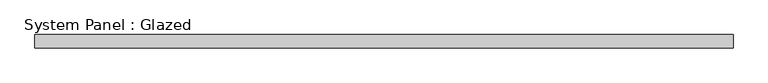
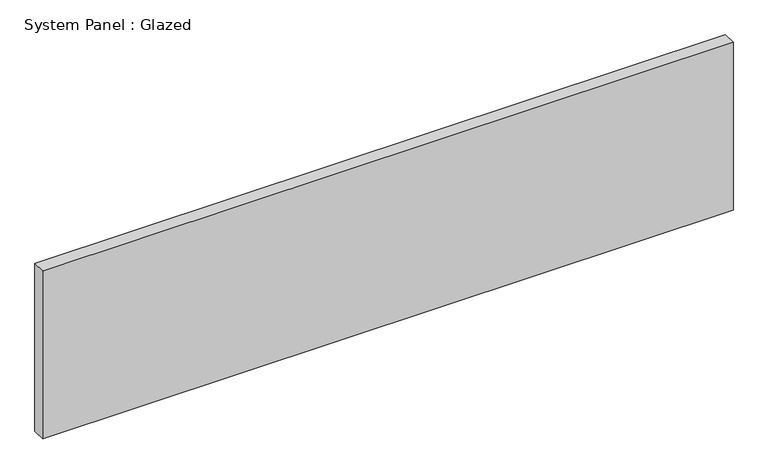
"""IFC4 building model written with IfcOpenShell, lengths in millimetres: plate geometry, System Panel : Glazed."""

from ifc_helpers import new_model, si_unit, origin, origin_with_axes, place, context, project, spatial, polyline, outline, extrude, source, transform, mapped, element, save


def system_panel_glazed_7354da21(model_context):
    return source(origin(), model_context, "Body", "SweptSolid", [
        extrude(outline(polyline([(666.7499999, -44.45), (-666.7499999, -44.45), (-666.7499999, -19.05), (666.7499999, -19.05), (666.7499999, -44.45)])), origin_with_axes(), (0.0, 0.0, 1.0), 342.9),
    ])


if __name__ == "__main__":
    model = new_model("IFC4")
    model_context = context("Model", 3, world=origin())
    ifc_project = project(units=[si_unit("LENGTHUNIT", "METRE", prefix="MILLI")], contexts=[model_context])
    site = spatial("IfcSite", under=ifc_project)
    building = spatial("IfcBuilding", under=site)
    placement = place(None, origin())
    system_panel_glazed_shape = system_panel_glazed_7354da21(model_context)
    element("IfcPlate", 1, ObjectType="System Panel : Glazed", at=placement, inside=building, context=model_context, shape_type="MappedRepresentation", body=[
        mapped(system_panel_glazed_shape, transform((0.0, 0.0, 0.0), x_axis=(1.0, 0.0, 0.0), y_axis=(0.0, 1.0, 0.0), z_axis=(0.0, 0.0, 1.0))),
    ])
    save(model, "model.ifc")

# Revit data of these elements
# Type "System Panel : Glazed"
#   Construction Type Id = "GSP4R"
#   Analytic Construction = "1/8 in Pilkington single glazing"
#   Visual Light Transmittance = 0.9
#   Solar Heat Gain Coefficient = 0.86
#   Heat Transfer Coefficient (U) = 1.18115 BTU/(h·ft²·°F)
#   Define Thermal Properties by = 1
# Element 1 (IfcPlate, "System Panel : Glazed")
#   Materials on its faces: "glass panel 223"
# Materials
#   "glass panel 223": class "Generic", colour RGB 120 120 120, transparency 0, Cost = 0
